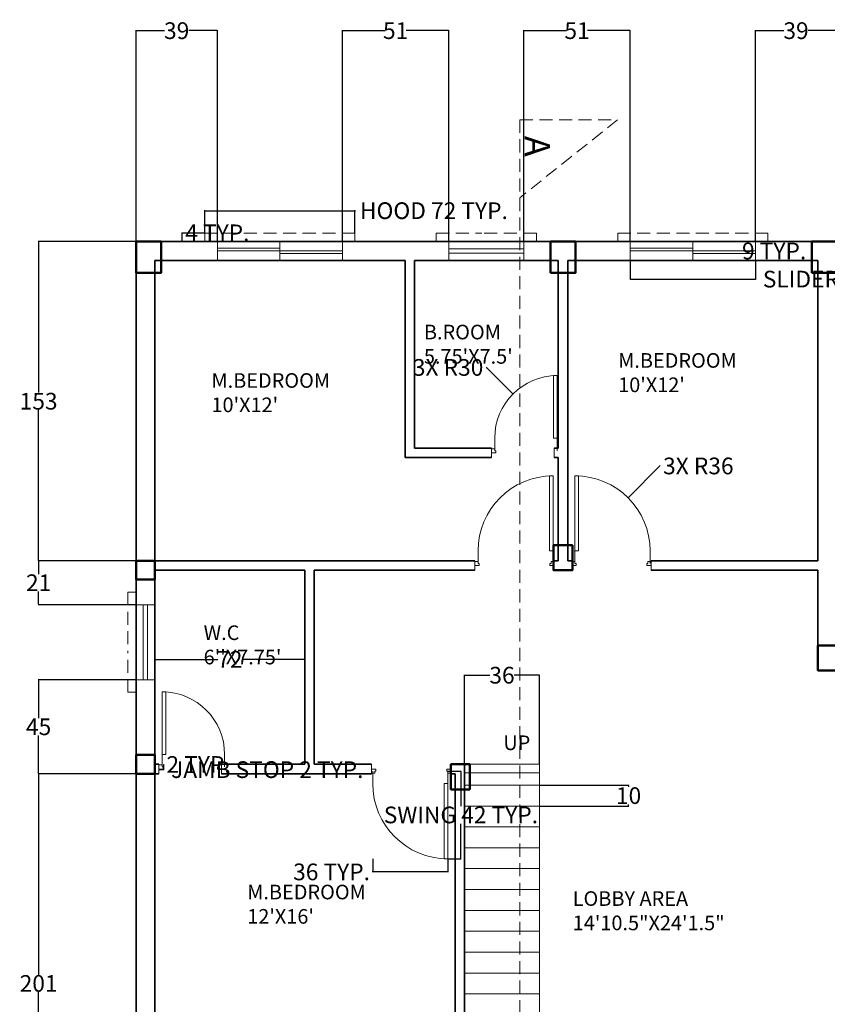
# Model space of a CAD drawing. Units: inches. Extents: x 683 to 1299, y -12 to 932.
# Tile 2 of 3: x 683 to 1070, y 460 to 932. Entities that reach past the tile are written whole.
import ezdxf

# ---------------------------------------------------------------- set-up
doc = ezdxf.new("R2010")
doc.units = ezdxf.units.IN
doc.header["$LTSCALE"] = 25
doc.header["$MEASUREMENT"] = 0
doc.linetypes.add('HIDDEN', pattern=[0.375, 0.25, -0.125])
for name, color, linetype, lineweight in [('A-ANNO-DIMS', 2, 'Continuous', 18), ('A-ANNO-SECT', 7, 'HIDDEN', 18), ('A-ANNO-TEXT', 6, 'Continuous', 25), ('A-AREA-IDEN', 6, 'Continuous', 18), ('A-COLS', 1, 'Continuous', 50), ('A-FLOR-STRS-HIDN', 5, 'HIDDEN', 18), ('A-GLAZ-OVHD', 7, 'HIDDEN', 13), ('A-WALL', 7, 'Continuous', 35)]:
    doc.layers.add(name, color=color, linetype=linetype, lineweight=lineweight)
doc.layers.add('A-DOOR', color=41, linetype='Continuous', lineweight=18, true_color=0xf4ee51)
doc.layers.add('A-GLAZ', color=41, linetype='Continuous', lineweight=18, true_color=0xf4ee51)
doc.styles.get("Standard").update_dxf_attribs({"font": 'arial.ttf'})
doc.dimstyles.get("Standard").update_dxf_attribs({"dimtxt": 8, "dimasz": 0.18, "dimexe": 0.18, "dimexo": 0.0625, "dimgap": 0.09, "dimtad": 0, "dimtih": 1, "dimtoh": 1, "dimdec": 1, "dimzin": 0, "dimdsep": 46, "dimlunit": 3, "dimtxsty": 'Standard', "dimcen": 0.09, "dimadec": 0, "dimazin": 0, "dimtfac": 1, "dimtdec": 1, "dimtofl": 0, "dimtmove": 0, "dimatfit": 3, "dimfxl": 1, "dimtolj": 1, "dimtzin": 0, "dimarcsym": 0})

# ---------------------------------------------------------------- blocks, each defined once
blk = doc.blocks.new('DOOR-SWING-36IN')
for p, q in [((0, 6), (0, 0)), ((36, 6), (36, 0))]:
    blk.add_line(p, q)
blk.add_lwpolyline([(0, 6), (0, 42), (1.75, 42), (1.75, 6)], close=True)
blk.add_arc((0, 6), 36, 0, 90)
blk = doc.blocks.new('DOOR-SWING-30IN')
for p, q in [((0, 6), (0, 0)), ((30, 6), (30, 0))]:
    blk.add_line(p, q)
blk.add_lwpolyline([(30, 6), (30, 36), (28.25, 36), (28.25, 6)], close=True)
blk.add_arc((30, 6), 30, 90, 180)
blk = doc.blocks.new('DOOR-JAMB-STOP')
for p, q in [((0, 2), (0, 0)), ((0, 2), (1.5, 2)), ((0, 0), (2, 0)), ((1.5, 1), (1.5, 2)), ((2, 1), (1.5, 1)), ((2, 0), (2, 1))]:
    blk.add_line(p, q)
blk = doc.blocks.new('WIN-SLIDER-60IN')
for p, q in [((60, 9), (0, 9)), ((0, 9), (0, 0)), ((30, 9), (30, 0)), ((60, 0), (60, 9)), ((0, 0), (60, 0)), ((30, 0), (60, 0))]:
    blk.add_line(p, q)
for points in [[(30, 4.5), (0, 4.5), (0, 5.76), (30, 5.76)], [(60, 3.24), (30, 3.24), (30, 4.5), (60, 4.5)]]:
    blk.add_lwpolyline(points, close=True)
blk = doc.blocks.new('WIN-36IN')
for p, q in [((36, 9), (0, 9)), ((0, 9), (0, 0)), ((0, 5.5), (36, 5.5)), ((36, 0), (36, 9)), ((0, 3.5), (36, 3.5)), ((0, 0), (36, 0))]:
    blk.add_line(p, q)
blk = doc.blocks.new('COLUMN-12X15IN')
blk.add_lwpolyline([(0, 0), (12, 0), (12, 15), (0, 15)], close=True)
blk = doc.blocks.new('COLUMN-12X9IN')
blk.add_lwpolyline([(0, 9), (0, 0), (12, 0), (12, 9)], close=True)
blk = doc.blocks.new('COLUMN-9X9IN')
blk.add_lwpolyline([(0, 0), (9, 0), (9, 9), (0, 9)], close=True)
blk = doc.blocks.new('WIN-HOOD-60IN')
for p, q in [((0, 0), (0, 4)), ((0, 4), (50.93, 4)), ((72, 4), (50.93, 4)), ((72, 0), (72, 4))]:
    blk.add_line(p, q)
blk = doc.blocks.new('*D12')
at = {"layer": 'A-ANNO-DIMS', "color": 0, "lineweight": -2, "ltscale": 25, "transparency": 16777216}
for p, q in [((749.97, 572.79), (749.97, 572.37)), ((750.15, 572.55), (751.79, 572.55)), ((751.97, 572.79), (751.97, 572.37)), ((751.97, 572.55), (752.15, 572.55))]:
    blk.add_line(p, q, dxfattribs=at)
at = {"layer": 'A-ANNO-DIMS', "color": 0, "ltscale": 25, "transparency": 16777216}
for points in [[(750.15, 572.58), (750.15, 572.52), (749.97, 572.55)], [(751.79, 572.58), (751.79, 572.52), (751.97, 572.55)]]:
    blk.add_solid(points, dxfattribs=at)
at = {"layer": 'Defpoints', "color": 0, "ltscale": 25, "transparency": 16777216}
for p in [(749.97, 572.85), (751.97, 572.85), (751.97, 572.55)]:
    blk.add_point(p, dxfattribs=at)
at = {"layer": 'A-ANNO-DIMS', "color": 0, "ltscale": 25, "transparency": 16777216, "insert": (801.91, 572.55), "char_height": 8, "attachment_point": 5}
blk.add_mtext('\\A1;JAMB STOP 2 TYP.', dxfattribs=at)
blk = doc.blocks.new('*D13')
at = {"layer": 'A-ANNO-DIMS', "color": 0, "lineweight": -2, "ltscale": 25, "transparency": 16777216}
for p, q in [((752.04, 574.85), (752.45, 574.85)), ((752.04, 572.85), (752.45, 572.85)), ((752.27, 574.85), (752.27, 575.03)), ((752.27, 575.03), (752.45, 575.03)), ((752.27, 573.03), (752.27, 574.67))]:
    blk.add_line(p, q, dxfattribs=at)
at = {"layer": 'A-ANNO-DIMS', "color": 0, "ltscale": 25, "transparency": 16777216}
for points in [[(752.24, 574.67), (752.3, 574.67), (752.27, 574.85)], [(752.24, 573.03), (752.3, 573.03), (752.27, 572.85)]]:
    blk.add_solid(points, dxfattribs=at)
at = {"layer": 'Defpoints', "color": 0, "ltscale": 25, "transparency": 16777216}
for p in [(751.97, 574.85), (751.97, 572.85), (752.27, 574.85)]:
    blk.add_point(p, dxfattribs=at)
at = {"layer": 'A-ANNO-DIMS', "color": 0, "ltscale": 25, "transparency": 16777216, "insert": (768.97, 575.03), "char_height": 8, "attachment_point": 5}
blk.add_mtext('\\A1;2 TYP.', dxfattribs=at)
blk = doc.blocks.new('*D18')
at = {"layer": 'A-ANNO-DIMS', "color": 0, "lineweight": -2, "ltscale": 25, "transparency": 16777216}
for p, q in [((975.97, 816.54), (975.97, 807.42)), ((1035.97, 816.54), (1035.97, 807.42)), ((976.15, 807.6), (1035.79, 807.6)), ((1035.97, 807.6), (1036.15, 807.6))]:
    blk.add_line(p, q, dxfattribs=at)
at = {"layer": 'A-ANNO-DIMS', "color": 0, "ltscale": 25, "transparency": 16777216}
for points in [[(976.15, 807.63), (976.15, 807.57), (975.97, 807.6)], [(1035.79, 807.63), (1035.79, 807.57), (1035.97, 807.6)]]:
    blk.add_solid(points, dxfattribs=at)
at = {"layer": 'Defpoints', "color": 0, "ltscale": 25, "transparency": 16777216}
for p in [(975.97, 816.6), (1035.97, 816.6), (1035.97, 807.6)]:
    blk.add_point(p, dxfattribs=at)
at = {"layer": 'A-ANNO-DIMS', "color": 0, "ltscale": 25, "transparency": 16777216, "insert": (1077.43, 807.6), "char_height": 8, "attachment_point": 5}
blk.add_mtext('\\A1;SLIDER 60 TYP.', dxfattribs=at)
blk = doc.blocks.new('*D19')
at = {"layer": 'A-ANNO-DIMS', "color": 0, "lineweight": -2, "ltscale": 25, "transparency": 16777216}
for p, q in [((1036.04, 825.6), (1045.15, 825.6)), ((1044.97, 825.42), (1044.97, 825.27)), ((1036.04, 816.6), (1045.15, 816.6)), ((1044.97, 816.78), (1044.97, 816.92))]:
    blk.add_line(p, q, dxfattribs=at)
at = {"layer": 'A-ANNO-DIMS', "color": 0, "ltscale": 25, "transparency": 16777216}
for points in [[(1044.94, 825.42), (1045, 825.42), (1044.97, 825.6)], [(1044.94, 816.78), (1045, 816.78), (1044.97, 816.6)]]:
    blk.add_solid(points, dxfattribs=at)
at = {"layer": 'Defpoints', "color": 0, "ltscale": 25, "transparency": 16777216}
for p in [(1035.97, 825.6), (1044.97, 825.6), (1035.97, 816.6)]:
    blk.add_point(p, dxfattribs=at)
at = {"layer": 'A-ANNO-DIMS', "color": 0, "ltscale": 25, "transparency": 16777216, "insert": (1044.97, 821.1), "char_height": 8, "attachment_point": 5}
blk.add_mtext('\\A1;9 TYP.', dxfattribs=at)
blk = doc.blocks.new('*D24')
at = {"layer": 'A-ANNO-DIMS', "color": 0, "lineweight": -2, "ltscale": 25, "transparency": 16777216}
for p, q in [((888.54, 571.85), (894.95, 571.85)), ((894.77, 571.67), (894.77, 555.08)), ((894.77, 530.03), (894.77, 546.62)), ((888.54, 529.85), (894.95, 529.85))]:
    blk.add_line(p, q, dxfattribs=at)
at = {"layer": 'A-ANNO-DIMS', "color": 0, "ltscale": 25, "transparency": 16777216}
for points in [[(894.74, 571.67), (894.8, 571.67), (894.77, 571.85)], [(894.74, 530.03), (894.8, 530.03), (894.77, 529.85)]]:
    blk.add_solid(points, dxfattribs=at)
at = {"layer": 'Defpoints', "color": 0, "ltscale": 25, "transparency": 16777216}
for p in [(888.47, 571.85), (888.47, 529.85), (894.77, 529.85)]:
    blk.add_point(p, dxfattribs=at)
at = {"layer": 'A-ANNO-DIMS', "color": 0, "ltscale": 25, "transparency": 16777216, "insert": (894.77, 550.85), "char_height": 8, "attachment_point": 5}
blk.add_mtext('\\A1;SWING 42 TYP.', dxfattribs=at)
blk = doc.blocks.new('*D25')
at = {"layer": 'A-ANNO-DIMS', "color": 0, "lineweight": -2, "ltscale": 25, "transparency": 16777216}
for p, q in [((852.47, 529.79), (852.47, 523.37)), ((888.47, 529.79), (888.47, 523.37)), ((852.47, 523.55), (852.29, 523.55)), ((888.29, 523.55), (852.65, 523.55))]:
    blk.add_line(p, q, dxfattribs=at)
at = {"layer": 'A-ANNO-DIMS', "color": 0, "ltscale": 25, "transparency": 16777216}
for points in [[(852.65, 523.58), (852.65, 523.52), (852.47, 523.55)], [(888.29, 523.58), (888.29, 523.52), (888.47, 523.55)]]:
    blk.add_solid(points, dxfattribs=at)
at = {"layer": 'Defpoints', "color": 0, "ltscale": 25, "transparency": 16777216}
for p in [(852.47, 529.85), (888.47, 529.85), (852.47, 523.55)]:
    blk.add_point(p, dxfattribs=at)
at = {"layer": 'A-ANNO-DIMS', "color": 0, "ltscale": 25, "transparency": 16777216, "insert": (832.74, 523.55), "char_height": 8, "attachment_point": 5}
blk.add_mtext('\\A1;36 TYP.', dxfattribs=at)
blk = doc.blocks.new('*D30')
at = {"layer": 'A-ANNO-DIMS', "color": 0, "lineweight": -2, "ltscale": 25, "transparency": 16777216}
for p, q in [((771.97, 829.66), (771.97, 840.58)), ((772.15, 840.4), (843.79, 840.4)), ((843.97, 829.66), (843.97, 840.58)), ((843.97, 840.4), (844.15, 840.4))]:
    blk.add_line(p, q, dxfattribs=at)
at = {"layer": 'A-ANNO-DIMS', "color": 0, "ltscale": 25, "transparency": 16777216}
for points in [[(772.15, 840.43), (772.15, 840.37), (771.97, 840.4)], [(843.79, 840.43), (843.79, 840.37), (843.97, 840.4)]]:
    blk.add_solid(points, dxfattribs=at)
at = {"layer": 'Defpoints', "color": 0, "ltscale": 25, "transparency": 16777216}
for p in [(843.97, 840.4), (771.97, 829.6), (843.97, 829.6)]:
    blk.add_point(p, dxfattribs=at)
at = {"layer": 'A-ANNO-DIMS', "color": 0, "ltscale": 25, "transparency": 16777216, "insert": (881.81, 840.4), "char_height": 8, "attachment_point": 5}
blk.add_mtext('\\A1;HOOD 72 TYP.', dxfattribs=at)
blk = doc.blocks.new('*D31')
at = {"layer": 'A-ANNO-DIMS', "color": 0, "lineweight": -2, "ltscale": 25, "transparency": 16777216}
for p, q in [((771.91, 829.6), (760.99, 829.6)), ((761.17, 829.6), (761.17, 829.78)), ((761.17, 829.78), (761.35, 829.78)), ((761.17, 825.78), (761.17, 829.42)), ((771.91, 825.6), (760.99, 825.6))]:
    blk.add_line(p, q, dxfattribs=at)
at = {"layer": 'A-ANNO-DIMS', "color": 0, "ltscale": 25, "transparency": 16777216}
for points in [[(761.14, 829.42), (761.2, 829.42), (761.17, 829.6)], [(761.14, 825.78), (761.2, 825.78), (761.17, 825.6)]]:
    blk.add_solid(points, dxfattribs=at)
at = {"layer": 'Defpoints', "color": 0, "ltscale": 25, "transparency": 16777216}
for p in [(761.17, 829.6), (771.97, 829.6), (771.97, 825.6)]:
    blk.add_point(p, dxfattribs=at)
at = {"layer": 'A-ANNO-DIMS', "color": 0, "ltscale": 25, "transparency": 16777216, "insert": (777.97, 829.78), "char_height": 8, "attachment_point": 5}
blk.add_mtext('\\A1;4 TYP.', dxfattribs=at)
blk = doc.blocks.new('*D34')
at = {"layer": 'A-ANNO-DIMS', "color": 0, "lineweight": -2, "ltscale": 25, "transparency": 16777216}
for p, q in [((738.97, 825.66), (738.97, 926.85)), ((739.15, 926.67), (752.65, 926.67)), ((777.79, 926.67), (764.3, 926.67)), ((777.97, 825.66), (777.97, 926.85))]:
    blk.add_line(p, q, dxfattribs=at)
at = {"layer": 'A-ANNO-DIMS', "color": 0, "ltscale": 25, "transparency": 16777216}
for points in [[(739.15, 926.7), (739.15, 926.64), (738.97, 926.67)], [(777.79, 926.7), (777.79, 926.64), (777.97, 926.67)]]:
    blk.add_solid(points, dxfattribs=at)
at = {"layer": 'Defpoints', "color": 0, "ltscale": 25, "transparency": 16777216}
for p in [(777.97, 926.67), (738.97, 825.6), (777.97, 825.6)]:
    blk.add_point(p, dxfattribs=at)
at = {"layer": 'A-ANNO-DIMS', "color": 0, "ltscale": 25, "transparency": 16777216, "insert": (758.47, 926.67), "char_height": 8, "attachment_point": 5}
blk.add_mtext('\\A1;39', dxfattribs=at)
blk = doc.blocks.new('*D35')
at = {"layer": 'A-ANNO-DIMS', "color": 0, "lineweight": -2, "ltscale": 25, "transparency": 16777216}
for p, q in [((837.97, 825.66), (837.97, 926.85)), ((838.15, 926.67), (858.43, 926.67)), ((888.79, 926.67), (868.52, 926.67)), ((888.97, 825.66), (888.97, 926.85))]:
    blk.add_line(p, q, dxfattribs=at)
at = {"layer": 'A-ANNO-DIMS', "color": 0, "ltscale": 25, "transparency": 16777216}
for points in [[(838.15, 926.7), (838.15, 926.64), (837.97, 926.67)], [(888.79, 926.7), (888.79, 926.64), (888.97, 926.67)]]:
    blk.add_solid(points, dxfattribs=at)
at = {"layer": 'Defpoints', "color": 0, "ltscale": 25, "transparency": 16777216}
for p in [(888.97, 926.67), (837.97, 825.6), (888.97, 825.6)]:
    blk.add_point(p, dxfattribs=at)
at = {"layer": 'A-ANNO-DIMS', "color": 0, "ltscale": 25, "transparency": 16777216, "insert": (863.47, 926.67), "char_height": 8, "attachment_point": 5}
blk.add_mtext('\\A1;51', dxfattribs=at)
blk = doc.blocks.new('*D36')
at = {"layer": 'A-ANNO-DIMS', "color": 0, "lineweight": -2, "ltscale": 25, "transparency": 16777216}
for p, q in [((924.97, 825.66), (924.97, 926.85)), ((925.15, 926.67), (945.43, 926.67)), ((975.79, 926.67), (955.52, 926.67)), ((975.97, 825.66), (975.97, 926.85))]:
    blk.add_line(p, q, dxfattribs=at)
at = {"layer": 'A-ANNO-DIMS', "color": 0, "ltscale": 25, "transparency": 16777216}
for points in [[(925.15, 926.7), (925.15, 926.64), (924.97, 926.67)], [(975.79, 926.7), (975.79, 926.64), (975.97, 926.67)]]:
    blk.add_solid(points, dxfattribs=at)
at = {"layer": 'Defpoints', "color": 0, "ltscale": 25, "transparency": 16777216}
for p in [(975.97, 926.67), (924.97, 825.6), (975.97, 825.6)]:
    blk.add_point(p, dxfattribs=at)
at = {"layer": 'A-ANNO-DIMS', "color": 0, "ltscale": 25, "transparency": 16777216, "insert": (950.47, 926.67), "char_height": 8, "attachment_point": 5}
blk.add_mtext('\\A1;51', dxfattribs=at)
blk = doc.blocks.new('*D37')
at = {"layer": 'A-ANNO-DIMS', "color": 0, "lineweight": -2, "ltscale": 25, "transparency": 16777216}
for p, q in [((1035.97, 825.66), (1035.97, 926.85)), ((1036.15, 926.67), (1049.65, 926.67)), ((1074.79, 926.67), (1061.3, 926.67)), ((1074.97, 825.66), (1074.97, 926.85))]:
    blk.add_line(p, q, dxfattribs=at)
at = {"layer": 'A-ANNO-DIMS', "color": 0, "ltscale": 25, "transparency": 16777216}
for points in [[(1036.15, 926.7), (1036.15, 926.64), (1035.97, 926.67)], [(1074.79, 926.7), (1074.79, 926.64), (1074.97, 926.67)]]:
    blk.add_solid(points, dxfattribs=at)
at = {"layer": 'Defpoints', "color": 0, "ltscale": 25, "transparency": 16777216}
for p in [(1074.97, 926.67), (1035.97, 825.6), (1074.97, 825.6)]:
    blk.add_point(p, dxfattribs=at)
at = {"layer": 'A-ANNO-DIMS', "color": 0, "ltscale": 25, "transparency": 16777216, "insert": (1055.47, 926.67), "char_height": 8, "attachment_point": 5}
blk.add_mtext('\\A1;39', dxfattribs=at)
blk = doc.blocks.new('*D41')
at = {"layer": 'A-ANNO-DIMS', "color": 0, "lineweight": -2, "ltscale": 25, "transparency": 16777216}
for p, q in [((738.91, 570.6), (692.09, 570.6)), ((692.27, 570.42), (692.27, 474.27)), ((692.27, 369.78), (692.27, 465.92)), ((738.91, 369.6), (692.09, 369.6))]:
    blk.add_line(p, q, dxfattribs=at)
at = {"layer": 'A-ANNO-DIMS', "color": 0, "ltscale": 25, "transparency": 16777216}
for points in [[(692.24, 570.42), (692.3, 570.42), (692.27, 570.6)], [(692.24, 369.78), (692.3, 369.78), (692.27, 369.6)]]:
    blk.add_solid(points, dxfattribs=at)
at = {"layer": 'Defpoints', "color": 0, "ltscale": 25, "transparency": 16777216}
for p in [(692.27, 570.6), (738.97, 570.6), (738.97, 369.6)]:
    blk.add_point(p, dxfattribs=at)
at = {"layer": 'A-ANNO-DIMS', "color": 0, "ltscale": 25, "transparency": 16777216, "insert": (692.27, 470.1), "char_height": 8, "attachment_point": 5}
blk.add_mtext('\\A1;201', dxfattribs=at)
blk = doc.blocks.new('*D42')
at = {"layer": 'A-ANNO-DIMS', "color": 0, "lineweight": -2, "ltscale": 25, "transparency": 16777216}
for p, q in [((738.91, 615.6), (692.09, 615.6)), ((692.27, 615.42), (692.27, 597.26)), ((692.27, 570.78), (692.27, 588.94)), ((738.91, 570.6), (692.09, 570.6))]:
    blk.add_line(p, q, dxfattribs=at)
at = {"layer": 'A-ANNO-DIMS', "color": 0, "ltscale": 25, "transparency": 16777216}
for points in [[(692.24, 615.42), (692.3, 615.42), (692.27, 615.6)], [(692.24, 570.78), (692.3, 570.78), (692.27, 570.6)]]:
    blk.add_solid(points, dxfattribs=at)
at = {"layer": 'Defpoints', "color": 0, "ltscale": 25, "transparency": 16777216}
for p in [(692.27, 615.6), (738.97, 615.6), (738.97, 570.6)]:
    blk.add_point(p, dxfattribs=at)
at = {"layer": 'A-ANNO-DIMS', "color": 0, "ltscale": 25, "transparency": 16777216, "insert": (692.27, 593.1), "char_height": 8, "attachment_point": 5}
blk.add_mtext('\\A1;45', dxfattribs=at)
blk = doc.blocks.new('*D43')
at = {"layer": 'A-ANNO-DIMS', "color": 0, "lineweight": -2, "ltscale": 25, "transparency": 16777216}
for p, q in [((738.91, 672.6), (692.09, 672.6)), ((692.27, 672.42), (692.27, 666.21)), ((692.27, 651.78), (692.27, 657.99)), ((738.91, 651.6), (692.09, 651.6))]:
    blk.add_line(p, q, dxfattribs=at)
at = {"layer": 'A-ANNO-DIMS', "color": 0, "ltscale": 25, "transparency": 16777216}
for points in [[(692.24, 672.42), (692.3, 672.42), (692.27, 672.6)], [(692.24, 651.78), (692.3, 651.78), (692.27, 651.6)]]:
    blk.add_solid(points, dxfattribs=at)
at = {"layer": 'Defpoints', "color": 0, "ltscale": 25, "transparency": 16777216}
for p in [(692.27, 672.6), (738.97, 672.6), (738.97, 651.6)]:
    blk.add_point(p, dxfattribs=at)
at = {"layer": 'A-ANNO-DIMS', "color": 0, "ltscale": 25, "transparency": 16777216, "insert": (692.27, 662.1), "char_height": 8, "attachment_point": 5}
blk.add_mtext('\\A1;21', dxfattribs=at)
blk = doc.blocks.new('*D44')
at = {"layer": 'A-ANNO-DIMS', "color": 0, "lineweight": -2, "ltscale": 25, "transparency": 16777216}
for p, q in [((738.91, 825.6), (692.09, 825.6)), ((692.27, 825.42), (692.27, 753.28)), ((692.27, 672.78), (692.27, 744.92)), ((738.91, 672.6), (692.09, 672.6))]:
    blk.add_line(p, q, dxfattribs=at)
at = {"layer": 'A-ANNO-DIMS', "color": 0, "ltscale": 25, "transparency": 16777216}
for points in [[(692.24, 825.42), (692.3, 825.42), (692.27, 825.6)], [(692.24, 672.78), (692.3, 672.78), (692.27, 672.6)]]:
    blk.add_solid(points, dxfattribs=at)
at = {"layer": 'Defpoints', "color": 0, "ltscale": 25, "transparency": 16777216}
for p in [(692.27, 825.6), (738.97, 825.6), (738.97, 672.6)]:
    blk.add_point(p, dxfattribs=at)
at = {"layer": 'A-ANNO-DIMS', "color": 0, "ltscale": 25, "transparency": 16777216, "insert": (692.27, 749.1), "char_height": 8, "attachment_point": 5}
blk.add_mtext('\\A1;153', dxfattribs=at)
blk = doc.blocks.new('*D50')
at = {"layer": 'A-ANNO-DIMS', "color": 0, "lineweight": -2, "ltscale": 25, "transparency": 16777216}
for p, q in [((896.47, 575.16), (896.47, 617.98)), ((896.65, 617.8), (908.66, 617.8)), ((932.29, 617.8), (920.29, 617.8)), ((932.47, 575.16), (932.47, 617.98))]:
    blk.add_line(p, q, dxfattribs=at)
at = {"layer": 'A-ANNO-DIMS', "color": 0, "ltscale": 25, "transparency": 16777216}
for points in [[(896.65, 617.83), (896.65, 617.77), (896.47, 617.8)], [(932.29, 617.83), (932.29, 617.77), (932.47, 617.8)]]:
    blk.add_solid(points, dxfattribs=at)
at = {"layer": 'Defpoints', "color": 0, "ltscale": 25, "transparency": 16777216}
for p in [(932.47, 617.8), (896.47, 575.1), (932.47, 575.1)]:
    blk.add_point(p, dxfattribs=at)
at = {"layer": 'A-ANNO-DIMS', "color": 0, "ltscale": 25, "transparency": 16777216, "insert": (914.47, 617.8), "char_height": 8, "attachment_point": 5}
blk.add_mtext('\\A1;36', dxfattribs=at)
blk = doc.blocks.new('*D51')
at = {"layer": 'A-ANNO-DIMS', "color": 0, "lineweight": -2, "ltscale": 25, "transparency": 16777216}
for p, q in [((932.54, 565.1), (975.35, 565.1)), ((975.17, 564.92), (975.17, 564.27)), ((932.54, 555.1), (975.35, 555.1)), ((975.17, 555.28), (975.17, 555.92))]:
    blk.add_line(p, q, dxfattribs=at)
at = {"layer": 'A-ANNO-DIMS', "color": 0, "ltscale": 25, "transparency": 16777216}
for points in [[(975.14, 564.92), (975.2, 564.92), (975.17, 565.1)], [(975.14, 555.28), (975.2, 555.28), (975.17, 555.1)]]:
    blk.add_solid(points, dxfattribs=at)
at = {"layer": 'Defpoints', "color": 0, "ltscale": 25, "transparency": 16777216}
for p in [(932.47, 565.1), (932.47, 555.1), (975.17, 555.1)]:
    blk.add_point(p, dxfattribs=at)
at = {"layer": 'A-ANNO-DIMS', "color": 0, "ltscale": 25, "transparency": 16777216, "insert": (975.17, 560.1), "char_height": 8, "attachment_point": 5}
blk.add_mtext('\\A1;10', dxfattribs=at)
blk = doc.blocks.new('*D54')
at = {"layer": 'A-ANNO-DIMS', "color": 0, "lineweight": -2, "ltscale": 25, "transparency": 16777216}
for p, q in [((747.97, 668.04), (747.97, 625.22)), ((819.97, 668.04), (819.97, 625.22)), ((748.15, 625.4), (778.23, 625.4)), ((819.79, 625.4), (789.72, 625.4))]:
    blk.add_line(p, q, dxfattribs=at)
at = {"layer": 'A-ANNO-DIMS', "color": 0, "ltscale": 25, "transparency": 16777216}
for points in [[(748.15, 625.43), (748.15, 625.37), (747.97, 625.4)], [(819.79, 625.43), (819.79, 625.37), (819.97, 625.4)]]:
    blk.add_solid(points, dxfattribs=at)
at = {"layer": 'Defpoints', "color": 0, "ltscale": 25, "transparency": 16777216}
for p in [(747.97, 668.1), (819.97, 668.1), (747.97, 625.4)]:
    blk.add_point(p, dxfattribs=at)
at = {"layer": 'A-ANNO-DIMS', "color": 0, "ltscale": 25, "transparency": 16777216, "insert": (783.97, 625.4), "char_height": 8, "attachment_point": 5}
blk.add_mtext('\\A1;72', dxfattribs=at)
blk = doc.blocks.new('*D61')
at = {"layer": 'A-ANNO-DIMS', "color": 0, "lineweight": -2, "ltscale": 25, "transparency": 16777216}
for p, q in [((990.2, 718.08), (975.06, 702.93)), ((990.38, 718.08), (990.2, 718.08)), ((949.38, 677.35), (949.56, 677.35)), ((949.47, 677.26), (949.47, 677.44))]:
    blk.add_line(p, q, dxfattribs=at)
at = {"layer": 'A-ANNO-DIMS', "color": 0, "ltscale": 25, "transparency": 16777216}
blk.add_solid([(975.04, 702.95), (975.08, 702.91), (974.93, 702.81)], dxfattribs=at)
at = {"layer": 'Defpoints', "color": 0, "ltscale": 25, "transparency": 16777216}
for p in [(974.93, 702.81), (949.47, 677.35)]:
    blk.add_point(p, dxfattribs=at)
at = {"layer": 'A-ANNO-DIMS', "color": 0, "ltscale": 25, "transparency": 16777216, "insert": (1008.62, 718.08), "char_height": 8, "attachment_point": 5}
blk.add_mtext('\\A1;3X R36', dxfattribs=at)
blk = doc.blocks.new('*D62')
at = {"layer": 'A-ANNO-DIMS', "color": 0, "lineweight": -2, "ltscale": 25, "transparency": 16777216}
for p, q in [((906.85, 765.29), (907.03, 765.29)), ((907.03, 765.29), (919.63, 752.69)), ((940.88, 731.35), (941.06, 731.35)), ((940.97, 731.26), (940.97, 731.44))]:
    blk.add_line(p, q, dxfattribs=at)
at = {"layer": 'A-ANNO-DIMS', "color": 0, "ltscale": 25, "transparency": 16777216}
blk.add_solid([(919.65, 752.71), (919.61, 752.67), (919.76, 752.56)], dxfattribs=at)
at = {"layer": 'Defpoints', "color": 0, "ltscale": 25, "transparency": 16777216}
for p in [(919.76, 752.56), (940.97, 731.35)]:
    blk.add_point(p, dxfattribs=at)
at = {"layer": 'A-ANNO-DIMS', "color": 0, "ltscale": 25, "transparency": 16777216, "insert": (888.63, 765.29), "char_height": 8, "attachment_point": 5}
blk.add_mtext('\\A1;3X R30', dxfattribs=at)

msp = doc.modelspace()

# ---------------------------------------------------------------- linework, layer by layer
at = {"layer": 'A-ANNO-SECT'}
for p, q in [((923.068, 883.972), (923.068, 36.355)), ((923.068, 883.972), (969.927, 883.972)), ((969.927, 883.972), (923.068, 846.632))]:
    msp.add_line(p, q, dxfattribs=at)
at = {"layer": 'A-COLS'}
msp.add_line((1065.973, 620.099), (1074.973, 620.099), dxfattribs=at)
at = {"layer": 'A-DOOR'}
for p, q in [((909.473, 726.599), (909.473, 722.099)), ((939.473, 726.599), (939.473, 722.099)), ((901.473, 672.599), (901.473, 668.099)), ((939.473, 672.599), (939.473, 668.099)), ((947.973, 672.599), (947.973, 668.099)), ((985.973, 672.599), (985.973, 668.099)), ((749.973, 575.099), (749.973, 570.599)), ((779.973, 575.099), (779.973, 570.599)), ((851.973, 570.599), (851.973, 575.099)), ((889.973, 570.599), (889.973, 575.099))]:
    msp.add_line(p, q, dxfattribs=at)
at = {"layer": 'A-FLOR-STRS-HIDN', "ltscale": 25}
for p, q in [((932.473, 575.099), (896.473, 575.099)), ((932.473, 571.099), (896.473, 571.099)), ((932.473, 575.099), (932.473, 378.599)), ((932.473, 565.099), (896.473, 565.099)), ((932.473, 565.099), (896.473, 565.099)), ((932.473, 565.099), (896.473, 565.099)), ((932.473, 555.099), (896.473, 555.099)), ((932.473, 545.099), (896.473, 545.099)), ((932.473, 535.099), (896.473, 535.099)), ((932.473, 525.099), (896.473, 525.099)), ((932.473, 515.099), (896.473, 515.099)), ((932.473, 505.099), (896.473, 505.099)), ((932.473, 495.099), (896.473, 495.099)), ((932.473, 485.099), (896.473, 485.099)), ((932.473, 475.099), (896.473, 475.099)), ((932.473, 465.099), (896.473, 465.099))]:
    msp.add_line(p, q, dxfattribs=at)
at = {"layer": 'A-GLAZ'}
for p, q in [((777.973, 825.599), (771.973, 825.599)), ((837.973, 825.599), (777.973, 825.599)), ((837.973, 825.599), (777.973, 825.599)), ((837.973, 825.599), (843.973, 825.599)), ((888.973, 825.599), (882.973, 825.599)), ((924.973, 825.599), (930.973, 825.599)), ((975.973, 825.599), (969.973, 825.599)), ((1035.973, 825.599), (975.973, 825.599)), ((975.973, 825.599), (975.973, 816.599)), ((1035.973, 816.599), (1035.973, 825.599)), ((1035.973, 825.599), (1041.973, 825.599)), ((906.973, 816.599), (924.973, 816.599)), ((975.973, 816.599), (1035.973, 816.599)), ((1005.973, 816.599), (1035.973, 816.599)), ((738.973, 651.599), (738.973, 657.599)), ((747.973, 651.599), (738.973, 651.599)), ((738.973, 651.599), (738.973, 615.599)), ((742.473, 651.599), (742.473, 615.599)), ((744.473, 651.599), (744.473, 615.599)), ((747.973, 621.599), (747.973, 651.599)), ((747.973, 615.599), (747.973, 621.599)), ((738.973, 615.599), (747.973, 615.599)), ((738.973, 615.599), (738.973, 609.599))]:
    msp.add_line(p, q, dxfattribs=at)
at = {"layer": 'A-GLAZ-OVHD'}
for p, q in [((882.973, 825.599), (882.973, 829.599)), ((882.973, 829.599), (904.757, 829.599)), ((930.973, 829.599), (904.757, 829.599)), ((930.973, 825.599), (930.973, 829.599)), ((738.973, 657.599), (734.973, 657.599)), ((734.973, 657.599), (734.973, 628.84)), ((734.973, 609.599), (734.973, 628.84)), ((738.973, 609.599), (734.973, 609.599))]:
    msp.add_line(p, q, dxfattribs=at)
at = {"layer": 'A-WALL'}
for p, q in [((738.973, 825.599), (1074.973, 825.599)), ((738.973, 825.599), (738.973, 369.599)), ((747.973, 816.599), (747.973, 672.599)), ((747.973, 816.599), (867.973, 816.599)), ((867.973, 816.599), (867.973, 722.099)), ((872.473, 816.599), (872.473, 726.599)), ((872.473, 816.599), (941.473, 816.599)), ((941.473, 816.599), (941.473, 726.599)), ((945.973, 816.599), (945.973, 672.599)), ((945.973, 816.599), (1065.973, 816.599)), ((1065.973, 816.599), (1065.973, 672.599)), ((867.973, 722.099), (909.473, 722.099)), ((872.473, 726.599), (909.473, 726.599)), ((939.473, 726.599), (941.473, 726.599)), ((939.473, 722.099), (941.473, 722.099)), ((941.473, 722.099), (941.473, 672.599)), ((747.973, 672.599), (867.973, 672.599)), ((747.973, 672.599), (901.473, 672.599)), ((939.473, 672.599), (941.473, 672.599)), ((945.973, 672.599), (947.973, 672.599)), ((985.973, 672.599), (1065.973, 672.599)), ((747.973, 668.099), (819.973, 668.099)), ((747.973, 668.099), (747.973, 575.099)), ((819.973, 668.099), (819.973, 575.099)), ((824.473, 668.099), (901.473, 668.099)), ((824.473, 668.099), (824.473, 575.099)), ((824.473, 668.099), (872.473, 668.099)), ((939.473, 668.099), (947.973, 668.099)), ((945.973, 668.099), (947.973, 668.099)), ((985.973, 668.099), (1065.973, 668.099)), ((985.973, 668.099), (1065.973, 668.099)), ((1065.973, 668.099), (1065.973, 620.099)), ((747.973, 575.099), (749.973, 575.099)), ((779.973, 575.099), (819.973, 575.099)), ((824.473, 575.099), (851.973, 575.099)), ((889.973, 575.099), (896.473, 575.099)), ((896.473, 575.099), (896.473, 378.599)), ((747.973, 570.599), (749.973, 570.599)), ((747.973, 570.599), (747.973, 378.599)), ((779.973, 570.599), (851.973, 570.599)), ((889.973, 570.599), (891.973, 570.599)), ((891.973, 570.599), (891.973, 378.599))]:
    msp.add_line(p, q, dxfattribs=at)

# ---------------------------------------------------------------- block references
at = {"layer": 'A-COLS'}
for name, p in [('COLUMN-12X15IN', (738.973, 810.599)), ('COLUMN-12X15IN', (937.716, 810.599)), ('COLUMN-12X15IN', (1062.973, 810.599)), ('COLUMN-9X9IN', (738.973, 663.599)), ('COLUMN-9X9IN', (738.973, 570.599))]:
    msp.add_blockref(name, p, dxfattribs=at)
for p, rotation in [((939.223, 680.099), 270.0000000000006), ((1065.973, 632.099), 270.0000000000001), ((889.973, 575.099), 269.9999999999997)]:
    msp.add_blockref('COLUMN-12X9IN', p, dxfattribs=dict(at, rotation=rotation))
at = {"layer": 'A-DOOR'}
for name, p in [('DOOR-SWING-30IN', (910.973, 725.349)), ('DOOR-JAMB-STOP', (909.473, 724.349)), ('DOOR-SWING-36IN', (949.473, 671.349)), ('DOOR-JAMB-STOP', (901.473, 670.349)), ('DOOR-JAMB-STOP', (947.973, 670.349)), ('DOOR-JAMB-STOP', (749.973, 572.849))]:
    msp.add_blockref(name, p, dxfattribs=at)
at = {"layer": 'A-DOOR', "extrusion": (0, 0, -1), "zscale": -1}
for name, p in [('DOOR-SWING-36IN', (-938.973, 671.349)), ('DOOR-JAMB-STOP', (-939.473, 670.349)), ('DOOR-JAMB-STOP', (-985.973, 670.349)), ('DOOR-SWING-30IN', (-781.473, 573.849)), ('DOOR-JAMB-STOP', (-779.973, 572.849))]:
    msp.add_blockref(name, p, dxfattribs=at)
at = {"layer": 'A-DOOR', "extrusion": (0, 0, -1), "zscale": -1, "rotation": 180}
msp.add_blockref('DOOR-JAMB-STOP', (-851.973, 572.849), dxfattribs=at)
at = {"layer": 'A-DOOR', "rotation": 180}
for name, p in [('DOOR-SWING-36IN', (888.473, 571.849)), ('DOOR-JAMB-STOP', (889.973, 572.849))]:
    msp.add_blockref(name, p, dxfattribs=at)
at = {"layer": 'A-GLAZ'}
for name, p in [('WIN-SLIDER-60IN', (777.973, 816.599)), ('WIN-36IN', (888.973, 816.599)), ('WIN-SLIDER-60IN', (975.973, 816.599))]:
    msp.add_blockref(name, p, dxfattribs=at)
at = {"layer": 'A-GLAZ-OVHD'}
for p in [(771.973, 825.599), (969.973, 825.599)]:
    msp.add_blockref('WIN-HOOD-60IN', p, dxfattribs=at)

# ---------------------------------------------------------------- texts
at = {"layer": 'A-ANNO-SECT', "ltscale": 25, "insert": (937.421, 876.223), "char_height": 12, "attachment_point": 1, "rotation": 270}
msp.add_mtext_dynamic_manual_height_columns('A', width=16.69857, gutter_width=1, heights=[0], dxfattribs=at)
at = {"layer": 'A-ANNO-TEXT', "ltscale": 25, "insert": (915.108, 588.927), "char_height": 7, "attachment_point": 1}
msp.add_mtext_dynamic_manual_height_columns('UP', width=117.16603, gutter_width=1, heights=[0], dxfattribs=at)
at = {"layer": 'A-AREA-IDEN', "ltscale": 25, "char_height": 7, "attachment_point": 1}
for s, insert in [("B.ROOM\\P5.75'X7.5'", (877.028, 785.743)), ("M.BEDROOM\\P10'X12'", (970.181, 772.137)), ("M.BEDROOM\\P10'X12'", (775.157, 762.533)), ("W.C \\P6''X7.75'", (771.404, 641.667)), ("M.BEDROOM\\P12'X16'", (792.312, 517.405)), ('LOBBY AREA\\P14\'10.5"X24\'1.5"', (948.383, 514.27))]:
    msp.add_mtext_dynamic_manual_height_columns(s, width=117.16603, gutter_width=1, heights=[0], dxfattribs=dict(at, insert=insert))

# ---------------------------------------------------------------- dimensions: what is measured, and where the dimension line sits
at = {"layer": 'A-ANNO-DIMS', "ltscale": 25}
for base, p1, p2, picture, middle in [((777.973, 926.672), (738.973, 825.599), (777.973, 825.599), '*D34', (758.473, 926.672)), ((888.973, 926.672), (837.973, 825.599), (888.973, 825.599), '*D35', (863.473, 926.672)), ((975.973, 926.672), (924.973, 825.599), (975.973, 825.599), '*D36', (950.473, 926.672)), ((1074.973, 926.672), (1035.973, 825.599), (1074.973, 825.599), '*D37', (1055.473, 926.672)), ((932.473, 617.799), (896.473, 575.099), (932.473, 575.099), '*D50', (914.473, 617.799))]:
    dim = msp.add_linear_dim(base=base, p1=p1, p2=p2, dimstyle='Standard', override={"dimdec": 0, "dimlfac": 1, "dimrnd": 0, "dimzin": 0, "dimdsep": 46, "dimlunit": 2}, dxfattribs=at)
    dim.commit()
    dim.dimension.update_dxf_attribs({"geometry": picture, "text_midpoint": middle})
for base, p1, p2, text, picture, middle in [((843.973, 840.399), (771.973, 829.599), (843.973, 829.599), 'HOOD <> TYP.', '*D30', (881.815, 840.399)), ((1035.973, 807.599), (975.973, 816.599), (1035.973, 816.599), 'SLIDER <> TYP.', '*D18', (1077.433, 807.599)), ((751.973, 572.549), (749.973, 572.849), (751.973, 572.849), 'JAMB STOP <> TYP.', '*D12', (801.91, 572.549))]:
    dim = msp.add_linear_dim(base=base, p1=p1, p2=p2, text=text, dimstyle='Standard', override={"dimdec": 0, "dimlfac": 1, "dimrnd": 0, "dimzin": 0, "dimdsep": 46, "dimlunit": 2}, dxfattribs=at)
    dim.commit()
    dim.dimension.update_dxf_attribs({"geometry": picture, "text_midpoint": middle})
for base, p1, p2, angle, text, picture, middle in [((761.173, 829.599), (771.973, 825.599), (771.973, 829.599), 90, '<> TYP.', '*D31', (777.967, 829.779)), ((1044.973, 825.599), (1035.973, 816.599), (1035.973, 825.599), 90, '<> TYP.', '*D19', (1044.973, 821.099)), ((752.273, 574.849), (751.973, 572.849), (751.973, 574.849), 90, '<> TYP.', '*D13', (768.974, 575.029)), ((894.773, 529.849), (888.473, 571.849), (888.473, 529.849), 270, 'SWING <> TYP.', '*D24', (894.773, 550.849)), ((852.473, 523.549), (888.473, 529.849), (852.473, 529.849), 180, '<> TYP.', '*D25', (832.735, 523.549))]:
    dim = msp.add_linear_dim(base=base, p1=p1, p2=p2, angle=angle, text=text, dimstyle='Standard', override={"dimdec": 0, "dimlfac": 1, "dimrnd": 0, "dimzin": 0, "dimdsep": 46, "dimlunit": 2}, dxfattribs=at)
    dim.commit()
    dim.dimension.update_dxf_attribs({"geometry": picture, "text_midpoint": middle})
for base, p1, p2, angle, picture, middle in [((692.273, 825.599), (738.973, 672.599), (738.973, 825.599), 90, '*D44', (692.273, 749.099)), ((692.273, 672.599), (738.973, 651.599), (738.973, 672.599), 90, '*D43', (692.273, 662.099)), ((747.973, 625.399), (819.973, 668.099), (747.973, 668.099), 180, '*D54', (783.973, 625.399)), ((692.273, 615.599), (738.973, 570.599), (738.973, 615.599), 90, '*D42', (692.273, 593.099)), ((692.273, 570.599), (738.973, 369.599), (738.973, 570.599), 90, '*D41', (692.273, 470.099)), ((975.173, 555.099), (932.473, 565.099), (932.473, 555.099), 270, '*D51', (975.173, 560.099))]:
    dim = msp.add_linear_dim(base=base, p1=p1, p2=p2, angle=angle, dimstyle='Standard', override={"dimdec": 0, "dimlfac": 1, "dimrnd": 0, "dimzin": 0, "dimdsep": 46, "dimlunit": 2}, dxfattribs=at)
    dim.commit()
    dim.dimension.update_dxf_attribs({"geometry": picture, "text_midpoint": middle})
for center, mpoint, picture, middle in [((940.973, 731.349), (919.76, 752.563), '*D62', (888.626, 765.291)), ((949.473, 677.349), (974.929, 702.805), '*D61', (1008.62, 718.078))]:
    dim = msp.add_radius_dim(center=center, mpoint=mpoint, text='3X <>', dimstyle='Standard', override={"dimdec": 0, "dimlfac": 1, "dimrnd": 0, "dimzin": 0, "dimdsep": 46, "dimlunit": 2}, dxfattribs=at)
    dim.commit()
    dim.dimension.update_dxf_attribs({"geometry": picture, "text_midpoint": middle, "dimtype": 164})

doc.saveas('drawing.dxf')
